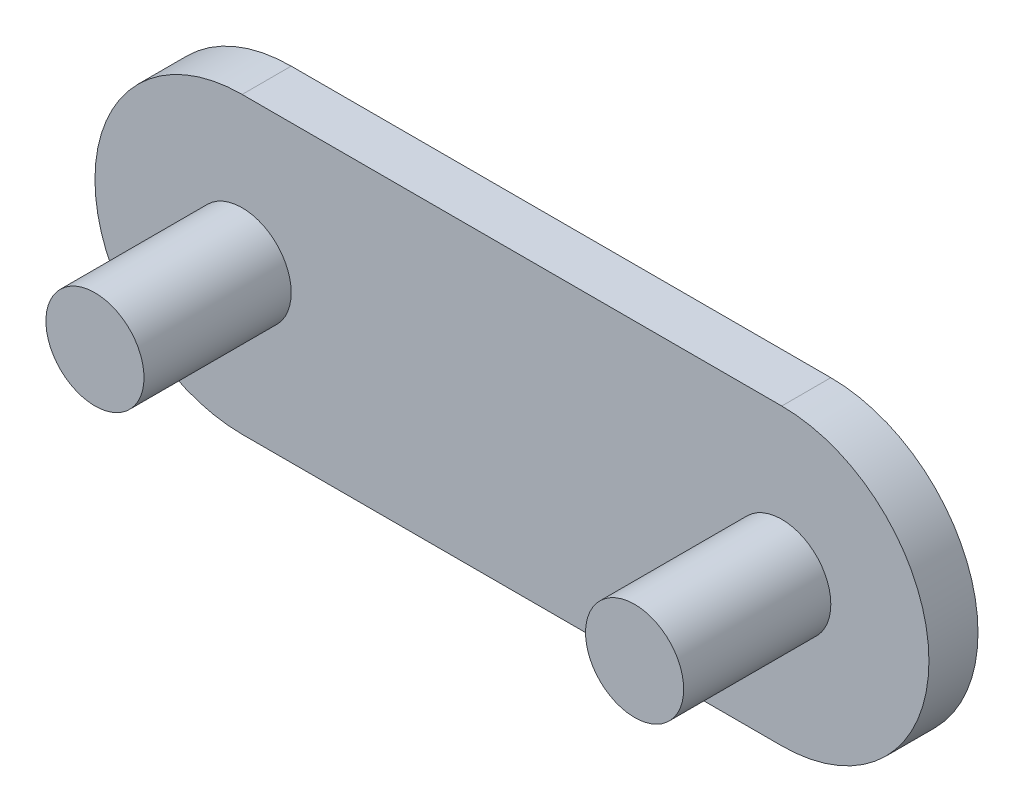
from build123d import *

# Parameters (mm, degrees)
BASE_PLATE_DEPTH     = 5
PIN_CIRCLES_SKETCH_R = 5
PINS_2X_10_DEPTH     = 15


with BuildPart() as part:
    # Plate Outline Sketch → Base Plate (new body)
    with BuildSketch(Plane.XY):
        with BuildLine():
            Line((-27.5, 15), (27.5, 15))
            ThreePointArc((27.5, 15), (42.5, 0), (27.5, -15))
            Line((27.5, -15), (-27.5, -15))
            ThreePointArc((-27.5, -15), (-42.5, 0), (-27.5, 15))
        make_face()
    extrude(amount=BASE_PLATE_DEPTH)

    # Pin Circles Sketch → Pins 2xØ10 (add)
    with BuildSketch(Plane.XY.offset(5)):
        with Locations((-27.5, 0)):
            Circle(PIN_CIRCLES_SKETCH_R)
        with Locations((27.5, 0)):
            Circle(PIN_CIRCLES_SKETCH_R)
    extrude(amount=PINS_2X_10_DEPTH)


solid = part.part
